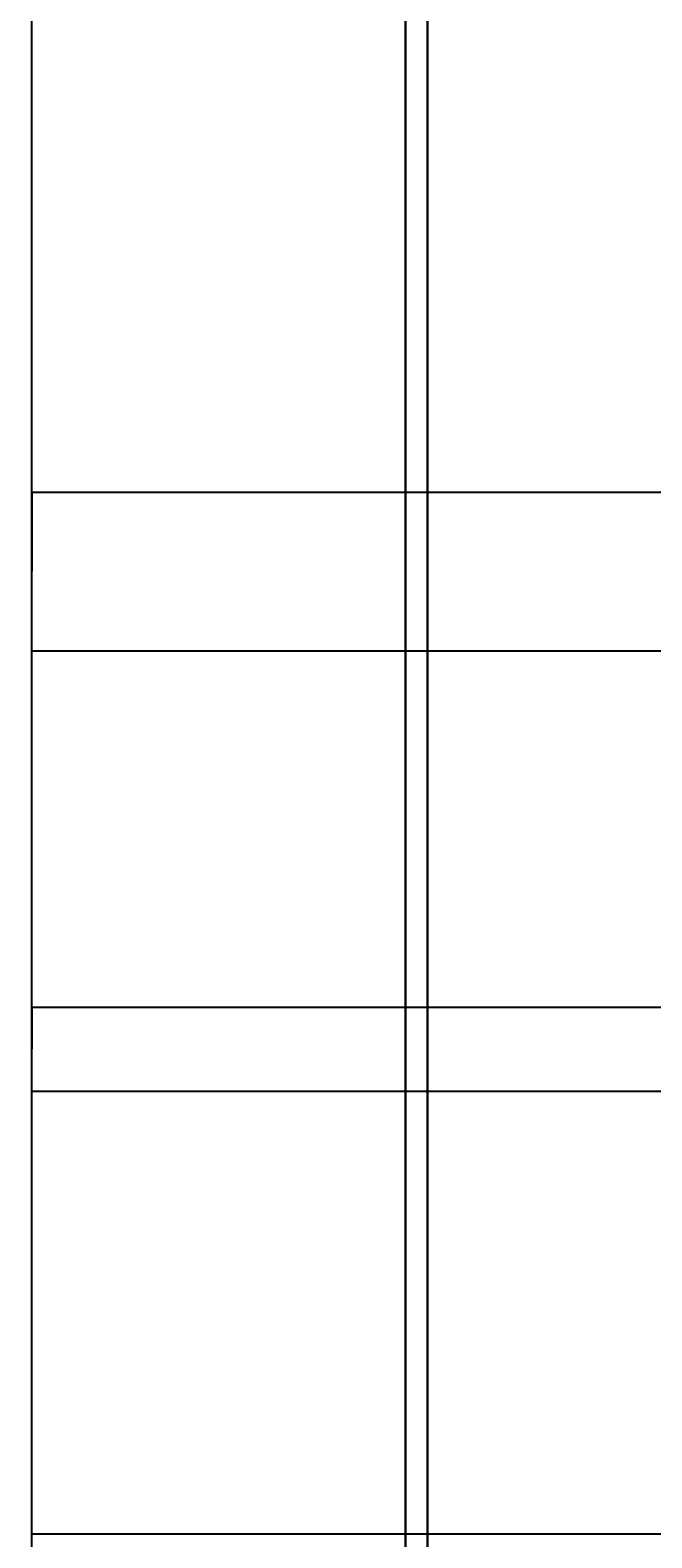
# Model space of a CAD drawing. Units: inches. Extents: x 2330 to 3943, y 1763 to 3461.
# Tile 2 of 40: x 2330 to 2472, y 2211 to 2554. Entities that reach past the tile are written whole.
import ezdxf

# ---------------------------------------------------------------- set-up
doc = ezdxf.new("R2010")
doc.units = ezdxf.units.IN
for name, color, linetype, lineweight in [('A-ANNO-DIMS', 2, 'Continuous', 18), ('C-PROP', 7, 'Continuous', 30), ('L-PLNT', 94, 'Continuous', 13)]:
    doc.layers.add(name, color=color, linetype=linetype, lineweight=lineweight)
doc.styles.get("Standard").update_dxf_attribs({"font": 'arial.ttf'})
doc.dimstyles.get("Standard").update_dxf_attribs({"dimtxt": 0.18, "dimasz": 0.18, "dimexe": 0.18, "dimexo": 0.0625, "dimgap": 0.09, "dimtad": 0, "dimtih": 1, "dimtoh": 1, "dimdec": 4, "dimzin": 0, "dimdsep": 46, "dimtxsty": 'Standard', "dimcen": 0.09, "dimadec": 0, "dimazin": 0, "dimtfac": 1, "dimtdec": 4, "dimtofl": 0, "dimtmove": 0, "dimatfit": 3, "dimfxl": 1, "dimtolj": 1, "dimtzin": 0, "dimarcsym": 0})

# ---------------------------------------------------------------- blocks, each defined once
blk = doc.blocks.new('*U15')
for points in [[(0, 60.64), (-3.051, 56.238), (-4.196, 52.815), (-5.34, 47.925), (-6.103, 45.969), (-11.062, 50.859), (-18.691, 52.326), (-20.98, 47.436), (-20.217, 43.524), (-20.598, 39.611), (-25.939, 43.035), (-27.846, 49.392), (-33.186, 52.326), (-30.516, 47.436), (-31.279, 43.035), (-30.135, 38.144), (-33.568, 35.21), (-40.815, 36.677), (-49.208, 38.144), (-46.919, 36.677), (-42.341, 31.787), (-42.341, 28.364), (-46.537, 27.386), (-55.692, 27.386), (-49.97, 22.006), (-54.548, 21.028), (-46.156, 14.671), (-51.496, 11.248), (-59.888, 11.248), (-55.692, 8.803), (-53.785, 5.38), (-57.218, 3.423), (-60.651, -1.467), (-61.033, -4.89), (-59.125, -3.423), (-54.548, -1.467), (-51.496, -4.401), (-53.022, -10.269), (-59.125, -15.16), (-49.208, -13.204), (-58.362, -24.451), (-48.445, -21.028), (-43.486, -22.495), (-43.104, -25.918), (-47.3, -31.298), (-43.104, -30.32), (-48.445, -39.611), (-38.527, -31.787), (-40.815, -36.188), (-32.423, -37.166), (-33.568, -43.523), (-35.475, -49.392), (-28.609, -44.99), (-23.65, -46.457), (-22.124, -51.837), (-21.743, -57.705), (-19.073, -52.326), (-15.639, -51.837), (-12.588, -58.683), (-11.062, -54.771), (-6.866, -49.392), (-6.866, -53.304), (-4.959, -48.414), (-1.907, -61.617), (-1.144, -51.348), (4.578, -59.172), (5.341, -54.282), (9.918, -56.727), (12.207, -60.639), (12.97, -47.925), (14.877, -44.501), (17.547, -47.436), (19.455, -52.815), (22.888, -60.639), (21.743, -49.392), (23.65, -46.457), (29.754, -47.925), (35.094, -52.326), (37.001, -53.793), (33.187, -46.457), (32.042, -41.567), (35.094, -39.122), (43.868, -40.589), (47.682, -42.056), (43.105, -36.188), (43.105, -33.743), (46.538, -31.298), (50.352, -32.765), (46.919, -26.407), (55.693, -22.495), (60.652, -22.984), (66.374, -22.006), (59.889, -20.05), (54.167, -18.094), (51.878, -15.649), (49.589, -12.225), (51.497, -10.269), (57.981, -9.78), (63.322, -7.335), (64.466, -2.934)], [(64.848, -2.934), (59.507, -5.379), (56.456, -4.401), (51.878, -2.445), (52.26, 0.978), (55.311, 3.912), (59.889, 5.869), (62.94, 11.248), (58.363, 10.27), (54.548, 10.27), (51.115, 11.248), (53.785, 15.649), (57.981, 18.094), (60.652, 19.561), (56.074, 19.561), (51.115, 17.605), (46.538, 19.072), (46.156, 22.496), (49.589, 27.386), (52.26, 34.721), (49.589, 33.743), (44.249, 30.32), (41.197, 32.276), (41.579, 37.655), (43.868, 42.546), (43.105, 46.947), (40.053, 44.013), (36.238, 40.589), (33.568, 42.057), (33.95, 45.969), (35.476, 52.815), (31.28, 49.392), (26.702, 46.947), (28.228, 50.859), (28.609, 61.129), (24.795, 54.282), (18.692, 50.859), (17.929, 57.706), (12.97, 50.859), (7.248, 57.706), (5.341, 53.304), (0, 60.64)]]:
    blk.add_lwpolyline(points)
blk.add_lwpolyline([(0.382, 1.956), (0, 0), (1.907, 0.489), (2.289, 1.467)], close=True)
blk = doc.blocks.new('*U12')
for p, q in [((-10.186, 53.64), (-13.084, 55.962)), ((0, 0), (-10.5, 57)), ((-9.099, 51.782), (-6.563, 55.962)), ((-8.737, 47.138), (-17.069, 52.711)), ((-7.65, 43.423), (-2.578, 49.46)), ((-5.839, 35.992), (4.667, 48.067)), ((-7.288, 39.707), (-21.778, 46.673)), ((-5.114, 27.632), (10.463, 46.673)), ((-5.114, 28.097), (-24.676, 40.636)), ((-2.941, 16.486), (8.652, 37.85)), ((-3.665, 19.273), (-27.574, 35.527)), ((27, 9), (48, 36)), ((27.127, 9.056), (31.112, 35.992)), ((44.153, 36.456), (45.239, 32.741)), ((16.259, 5.805), (23.142, 31.348)), ((22.055, 7.198), (27.489, 32.277)), ((31.836, 30.883), (32.561, 16.486)), ((35.096, 32.741), (37.27, 22.524)), ((38.719, 34.134), (41.979, 28.561)), ((43.791, 29.954), (51.036, 30.883)), ((-48.585, 21.131), (-49.309, 29.026)), ((-43.513, 28.561), (-42.427, 15.558)), ((-35.544, 28.097), (-24.314, 3.947)), ((-31.5, 4.5), (-52.5, 25.5)), ((-38.442, 26.239), (-34.819, 7.663)), ((-14.533, 2.09), (-30.834, 25.31)), ((-1.129, 6.734), (9.014, 26.704)), ((3.942, 1.625), (11.187, 24.381)), ((10.101, 3.483), (17.708, 26.239)), ((40.53, 25.775), (48.862, 24.846)), ((-24.314, 23.917), (-2.941, 13.7)), ((-47.498, 19.737), (-55.83, 18.344)), ((36.183, 19.737), (48.137, 17.88)), ((-40.615, 13.7), (-55.105, 10.913)), ((-20.691, 13.7), (-1.129, 4.876)), ((33.285, 16.486), (48.862, 10.913)), ((29.662, 12.307), (48.137, 6.269)), ((0, 0), (27, 9)), ((24.229, 7.663), (46.688, 1.625)), ((-33.37, 6.269), (-52.207, 5.34)), ((-28.299, 3.483), (-47.86, -5.805)), ((0, 0), (-31.5, 4.5)), ((11.187, 3.483), (30.749, -5.805)), ((18.07, 5.805), (35.096, -3.483)), ((-21.416, 3.018), (-38.079, -8.128)), ((-15.982, 2.09), (-30.11, -9.521)), ((0, 0), (-22.5, -19.5)), ((-6.563, 1.161), (-21.416, -8.128)), ((0, 0), (18, -22.5)), ((6.478, 1.625), (26.04, -8.592)), ((2.493, -3.019), (-1.491, -20.202)), ((1.769, -2.555), (24.229, -9.521)), ((-6.563, -5.805), (-19.967, -9.985)), ((-4.752, -3.483), (-3.665, -14.629)), ((5.029, -6.27), (2.131, -25.775)), ((-9.461, -8.592), (-6.201, -23.453)), ((7.565, -9.056), (32.198, -14.629)), ((-15.257, -12.772), (-30.11, -12.772)), ((-13.446, -11.378), (-8.737, -32.741)), ((9.014, -11.378), (3.58, -35.992)), ((-17.431, -15.094), (-42.789, -18.809)), ((-17.069, -15.094), (-12.721, -40.172)), ((14.085, -16.951), (6.478, -40.172)), ((12.274, -15.094), (36.907, -18.809)), ((-22.5, -19.5), (-37.5, -45)), ((-20.691, -18.345), (-17.793, -44.352)), ((16.259, -19.738), (36.183, -22.989)), ((-24.314, -21.596), (-42.427, -22.06)), ((-25.038, -23.918), (-22.865, -45.281)), ((18.07, -22.524), (8.289, -45.745)), ((18, -22.5), (27, -52.5)), ((18.433, -22.524), (40.53, -29.026)), ((-26.849, -26.24), (-40.253, -25.775)), ((19.157, -25.311), (38.719, -33.206)), ((-28.299, -29.026), (-42.789, -31.348)), ((20.244, -30.419), (15.897, -44.816)), ((-30.834, -34.135), (-42.427, -35.528)), ((-29.023, -30.884), (-27.936, -43.887)), ((21.331, -32.741), (39.081, -40.636)), ((-32.646, -36.921), (-31.921, -44.352)), ((-34.457, -39.708), (-40.978, -42.494)), ((22.78, -37.85), (19.519, -48.532)), ((22.78, -38.314), (34.372, -44.816)), ((24.591, -43.423), (30.749, -47.603)), ((24.591, -45.745), (23.142, -50.854)), ((26.764, -49.925), (28.213, -50.854))]:
    blk.add_line(p, q)
blk = doc.blocks.new('*D60')
at = {"layer": 'A-ANNO-DIMS', "color": 0, "lineweight": -2, "transparency": 16777216}
for p, q in [((2415.6, 3210.65), (2330.5, 3210.65)), ((2330.68, 3210.47), (2330.68, 2592.83)), ((2330.68, 1974.83), (2330.68, 2592.47)), ((2415.6, 1974.65), (2330.5, 1974.65))]:
    blk.add_line(p, q, dxfattribs=at)
at = {"layer": 'A-ANNO-DIMS', "color": 0, "transparency": 16777216}
for points in [[(2330.65, 3210.47), (2330.71, 3210.47), (2330.68, 3210.65)], [(2330.65, 1974.83), (2330.71, 1974.83), (2330.68, 1974.65)]]:
    blk.add_solid(points, dxfattribs=at)
at = {"layer": 'Defpoints', "color": 0, "transparency": 16777216}
for p in [(2330.68, 3210.65), (2415.66, 3210.65), (2415.66, 1974.65)]:
    blk.add_point(p, dxfattribs=at)
at = {"layer": 'A-ANNO-DIMS', "color": 0, "transparency": 16777216, "insert": (2330.68, 2592.65), "char_height": 0.18, "attachment_point": 5}
blk.add_mtext('\\A1;1236', dxfattribs=at)
blk = doc.blocks.new('*D62')
at = {"layer": 'A-ANNO-DIMS', "color": 0, "lineweight": -2, "transparency": 16777216}
for p, q in [((2475.6, 3162.65), (2330.5, 3162.65)), ((2330.68, 3162.47), (2330.68, 2687.58)), ((2330.68, 2212.33), (2330.68, 2687.22)), ((2475.6, 2212.15), (2330.5, 2212.15))]:
    blk.add_line(p, q, dxfattribs=at)
at = {"layer": 'A-ANNO-DIMS', "color": 0, "transparency": 16777216}
for points in [[(2330.65, 3162.47), (2330.71, 3162.47), (2330.68, 3162.65)], [(2330.65, 2212.33), (2330.71, 2212.33), (2330.68, 2212.15)]]:
    blk.add_solid(points, dxfattribs=at)
at = {"layer": 'Defpoints', "color": 0, "transparency": 16777216}
for p in [(2330.68, 3162.65), (2475.66, 3162.65), (2475.66, 2212.15)]:
    blk.add_point(p, dxfattribs=at)
at = {"layer": 'A-ANNO-DIMS', "color": 0, "transparency": 16777216, "insert": (2330.68, 2687.4), "char_height": 0.18, "attachment_point": 5}
blk.add_mtext('\\A1;950.5', dxfattribs=at)
blk = doc.blocks.new('*D78')
at = {"layer": 'A-ANNO-DIMS', "color": 0, "lineweight": -2, "transparency": 16777216}
for p, q in [((2717.6, 2448.65), (2330.5, 2448.65)), ((2330.68, 2448.47), (2330.68, 2430.83)), ((2330.68, 2412.83), (2330.68, 2430.47)), ((2717.6, 2412.65), (2330.5, 2412.65))]:
    blk.add_line(p, q, dxfattribs=at)
at = {"layer": 'A-ANNO-DIMS', "color": 0, "transparency": 16777216}
for points in [[(2330.65, 2448.47), (2330.71, 2448.47), (2330.68, 2448.65)], [(2330.65, 2412.83), (2330.71, 2412.83), (2330.68, 2412.65)]]:
    blk.add_solid(points, dxfattribs=at)
at = {"layer": 'Defpoints', "color": 0, "transparency": 16777216}
for p in [(2330.68, 2448.65), (2717.66, 2448.65), (2717.66, 2412.65)]:
    blk.add_point(p, dxfattribs=at)
at = {"layer": 'A-ANNO-DIMS', "color": 0, "transparency": 16777216, "insert": (2330.68, 2430.65), "char_height": 0.18, "attachment_point": 5}
blk.add_mtext('\\A1;36', dxfattribs=at)
blk = doc.blocks.new('*D80')
at = {"layer": 'A-ANNO-DIMS', "color": 0, "lineweight": -2, "transparency": 16777216}
for p, q in [((3166.6, 2331.7), (2330.5, 2331.7)), ((2330.68, 2331.52), (2330.68, 2322.36)), ((2330.68, 2312.83), (2330.68, 2321.99)), ((3166.6, 2312.65), (2330.5, 2312.65))]:
    blk.add_line(p, q, dxfattribs=at)
at = {"layer": 'A-ANNO-DIMS', "color": 0, "transparency": 16777216}
for points in [[(2330.65, 2331.52), (2330.71, 2331.52), (2330.68, 2331.7)], [(2330.65, 2312.83), (2330.71, 2312.83), (2330.68, 2312.65)]]:
    blk.add_solid(points, dxfattribs=at)
at = {"layer": 'Defpoints', "color": 0, "transparency": 16777216}
for p in [(2330.68, 2331.7), (3166.66, 2331.7), (3166.66, 2312.65)]:
    blk.add_point(p, dxfattribs=at)
at = {"layer": 'A-ANNO-DIMS', "color": 0, "transparency": 16777216, "insert": (2330.68, 2322.18), "char_height": 0.18, "attachment_point": 5}
blk.add_mtext('\\A1;19.046', dxfattribs=at)

msp = doc.modelspace()

# ---------------------------------------------------------------- linework, layer by layer
at = {"layer": 'C-PROP'}
for p, q in [((2415.6605, 3210.6524), (2415.6605, 1974.6524)), ((2420.6605, 3205.6524), (2420.6605, 1979.6524))]:
    msp.add_line(p, q, dxfattribs=at)

# ---------------------------------------------------------------- block references
at = {"layer": 'L-PLNT', "xscale": -1, "rotation": 279.1543537978463}
for name, p in [('*U15', (2477.6333, 2145.4094)), ('*U12', (2513.0823, 2155.9909))]:
    msp.add_blockref(name, p, dxfattribs=at)

# ---------------------------------------------------------------- dimensions: what is measured, and where the dimension line sits
at = {"layer": 'A-ANNO-DIMS'}
for base, p1, p2, override, picture, middle in [((2330.6824, 3210.6524), (2415.6605, 1974.6524), (2415.6605, 3210.6524), {"dimdec": 0, "dimlfac": 1, "dimrnd": 0, "dimzin": 0, "dimdsep": 46, "dimlunit": 2}, '*D60', (2330.6824, 2592.6524)), ((2330.6824, 3162.6524), (2475.6605, 2212.1524), (2475.6605, 3162.6524), {"dimdec": 1, "dimlfac": 1, "dimrnd": 0, "dimzin": 0, "dimdsep": 46, "dimlunit": 2}, '*D62', (2330.6824, 2687.4024)), ((2330.6824, 2448.6524), (2717.6605, 2412.6524), (2717.6605, 2448.6524), {"dimdec": 0, "dimlfac": 1, "dimrnd": 0, "dimzin": 0, "dimdsep": 46, "dimlunit": 2}, '*D78', (2330.6824, 2430.6524)), ((2330.6824, 2331.6982), (3166.6605, 2312.6524), (3166.6605, 2331.6982), {"dimdec": 3, "dimlfac": 1, "dimrnd": 0, "dimzin": 0, "dimdsep": 46, "dimlunit": 2}, '*D80', (2330.6824, 2322.1753))]:
    dim = msp.add_linear_dim(base=base, p1=p1, p2=p2, angle=90, dimstyle='Standard', override=override, dxfattribs=at)
    dim.commit()
    dim.dimension.update_dxf_attribs({"geometry": picture, "text_midpoint": middle})

doc.saveas('drawing.dxf')
